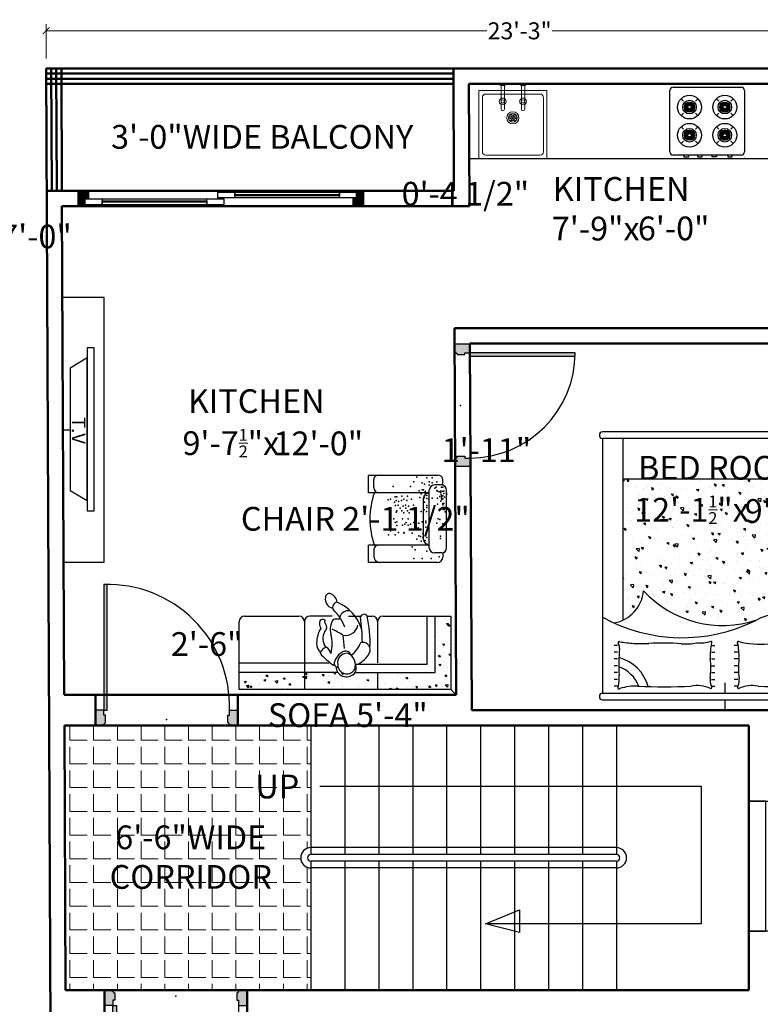
# Model space of a CAD drawing. Units: inches. Extents: x 4508 to 5907, y 877 to 1592.
# Tile 19 of 20: x 5566 to 5784, y 1298 to 1588. Entities that reach past the tile are written whole.
import ezdxf

# ---------------------------------------------------------------- set-up
doc = ezdxf.new("R2010")
doc.units = ezdxf.units.IN
doc.layers.get('DEFPOINTS').update_dxf_attribs({"color": 8})
for name, color, linetype, lineweight in [('A-ANNO-DIMS', 2, 'Continuous', 18), ('A-ANNO-TEXT', 7, 'Continuous', 25), ('A-DOOR', 4, 'Continuous', 25), ('A-EQPM', 6, 'Continuous', 25), ('A-FLOR-CASE', 30, 'Continuous', 25), ('A-FLOR-FIXT', 8, 'Continuous', 18), ('A-FLOR-PATT', 252, 'Continuous', 13), ('A-FLOR-STRS', 5, 'Continuous', 25), ('A-FURN', 24, 'Continuous', 18), ('A-WALL', 7, 'Continuous', 50)]:
    doc.layers.add(name, color=color, linetype=linetype, lineweight=lineweight)
doc.layers.add('doors & windows', color=30, linetype='Continuous')
doc.layers.add('furniture', color=24, linetype='Continuous')
doc.styles.get("Standard").update_dxf_attribs({"font": 'arial.ttf'})
doc.dimstyles.new('details', dxfattribs={"dimtxt": 5, "dimasz": 2, "dimexe": 2, "dimexo": 3, "dimgap": 1, "dimtad": 0, "dimdec": 1, "dimzin": 0, "dimdsep": 46, "dimlunit": 4, "dimtxsty": 'Standard', "dimblk": 'ARCHTICK', "dimcen": 3, "dimclrd": 256, "dimclre": 256, "dimclrt": 256, "dimadec": 0, "dimazin": 0, "dimtfac": 0.5, "dimtdec": 1, "dimtofl": 0, "dimtmove": 0, "dimatfit": 3, "dimldrblk": 'CLOSEDBLANK', "dimfxl": 2, "dimtolj": 1, "dimtzin": 0, "dimlwd": -1, "dimlwe": -1, "dimarcsym": 0})
doc.dimstyles.new('text', dxfattribs={"dimtxt": 7, "dimasz": 0, "dimexe": 3, "dimexo": 3, "dimgap": 0, "dimtad": 1, "dimtih": 1, "dimtoh": 1, "dimzin": 3, "dimdsep": 46, "dimlunit": 4, "dimtxsty": 'Standard', "dimblk": 'CLOSEDBLANK', "dimcen": 3, "dimse1": 1, "dimse2": 1, "dimsd1": 1, "dimsd2": 1, "dimclrd": 256, "dimclre": 256, "dimclrt": 256, "dimadec": 0, "dimazin": 0, "dimtfac": 0.5, "dimtofl": 0, "dimtmove": 0, "dimatfit": 3, "dimfxl": 3, "dimtolj": 1, "dimtzin": 0, "dimlwd": -1, "dimlwe": -1, "dimarcsym": 0})

# ---------------------------------------------------------------- blocks, each defined once
blk = doc.blocks.new('*D114')
at = {"layer": 'DEFPOINTS', "color": 0, "transparency": 16777216}
for p in [(5615.84, 1381.24), (5615.84, 1303.24), (5616.61, 1303.24)]:
    blk.add_point(p, dxfattribs=at)
at = {"layer": 'A-ANNO-DIMS', "color": 0, "transparency": 16777216, "insert": (5616.61, 1341.61), "char_height": 7, "attachment_point": 5}
blk.add_mtext('\\A1;6\'-6"WIDE \\PCORRIDOR', dxfattribs=at)
blk = doc.blocks.new('_ClosedBlank')
at = {"color": 0, "lineweight": -2}
for p, q in [((-1, 0.17), (0, 0)), ((-1, 0.17), (-1, -0.17)), ((0, 0), (-1, -0.17))]:
    blk.add_line(p, q, dxfattribs=at)
blk = doc.blocks.new('FD')
h = blk.add_hatch()
h.set_pattern_fill('ANSI31', color=256, style=0)
h.set_pattern_definition([(315, (2e-11, -5), (-0.0883883, -0.0883883), [])])
h.paths.add_polyline_path([(0, -4.5), (0, 0), (3, 0), (3, -2.5), (2, -2.5), (2, -4), (2, -4.5)])
h = blk.add_hatch()
h.set_pattern_fill('ANSI31', color=256, style=0)
h.set_pattern_definition([(135, (84, 0.5), (0.0883883, 0.0883883), [])])
h.paths.add_polyline_path([(84, 0), (84, -4.5), (81, -4.5), (81, -2), (82, -2), (82, -0.5), (82, 0)])
for p, q in [((0, -4.5), (0, 0)), ((0, 0), (84, 0)), ((84, 0), (84, -4.5)), ((0, -4.5), (84, -4.5))]:
    blk.add_line(p, q)
at = {"layer": 'doors & windows'}
for p, q in [((0, 0), (3, 0)), ((82, 0), (84, 0)), ((82, -2), (82, 0)), ((2, -2.5), (2, -4)), ((2, -2.5), (2, -4.5)), ((76.94, -1.25), (46.1, -1.25)), ((82, -2), (82, -0.5)), ((2, -4.5), (0, -4.5)), ((7.06, -3.25), (37.9, -3.25)), ((84, -4.5), (81, -4.5))]:
    blk.add_line(p, q, dxfattribs=at)
for points in [[(3, 0), (3, -2.5), (2, -2.5)], [(2, -4), (43, -4), (43, -2.5), (2, -2.5), (2, -4)], [(7.06, -2.5), (7.06, -4), (7.06, -3), (37.9, -3), (37.9, -4), (37.9, -2.5)], [(82, -0.5), (41, -0.5), (41, -2), (82, -2), (82, -0.5)], [(76.94, -2), (76.94, -0.5), (76.94, -1.5), (46.1, -1.5), (46.1, -0.5), (46.1, -2)], [(81, -4.5), (81, -2), (82, -2)]]:
    blk.add_lwpolyline(points, dxfattribs=at)
blk = doc.blocks.new('*D117')
at = {"layer": 'DEFPOINTS', "color": 0, "transparency": 16777216}
for p in [(5791.67, 1535.67), (5698.68, 1533.69), (5791.67, 1523.15)]:
    blk.add_point(p, dxfattribs=at)
at = {"layer": 'A-ANNO-DIMS', "color": 0, "transparency": 16777216, "insert": (5735.91, 1532.61), "char_height": 7, "attachment_point": 5}
blk.add_mtext('\\A1;       KITCHEN\\P7\'-9"x', dxfattribs=at)
blk = doc.blocks.new('*D118')
at = {"layer": 'DEFPOINTS', "color": 0, "transparency": 16777216}
for p in [(5748.26, 1569.42), (5758.87, 1569.42), (5754.78, 1497.42)]:
    blk.add_point(p, dxfattribs=at)
at = {"layer": 'A-ANNO-DIMS', "color": 0, "transparency": 16777216, "insert": (5758.87, 1526.82), "char_height": 7, "attachment_point": 5}
blk.add_mtext('\\A1;6\'-0"', dxfattribs=at)
blk = doc.blocks.new('stove')
at = {"layer": 'furniture'}
h = blk.add_hatch(dxfattribs=at)
h.set_pattern_fill('HEX', color=256, angle=180, style=0)
h.set_pattern_definition([(360, (22, 21.5), (1e-16, 0.2165064), [0.125, -0.25]), (120, (22, 21.5), (-0.1875, -0.1082532), [0.125, -0.25]), (60, (22.125, 21.5), (-0.1875, 0.1082532), [0.125, -0.25])])
h.paths.add_polyline_path([(5.36, 16.21, 1), (8.36, 16.21, 1)])
h.paths.add_polyline_path([(7.36, 16.21, -1), (6.36, 16.21, -1)], flags=16)
h = blk.add_hatch(dxfattribs=at)
h.set_pattern_fill('HEX', color=256, angle=180, style=0)
h.set_pattern_definition([(180, (2e-13, 21.5), (-1e-16, 0.2165064), [0.125, -0.25]), (60, (2e-13, 21.5), (0.1875, -0.1082532), [0.125, -0.25]), (120, (-0.125, 21.5), (0.1875, 0.1082532), [0.125, -0.25])])
h.paths.add_polyline_path([(13.64, 16.21, 1), (16.64, 16.21, 1)])
h.paths.add_polyline_path([(15.64, 16.21, -1), (14.64, 16.21, -1)], flags=16)
h = blk.add_hatch(dxfattribs=at)
h.set_pattern_fill('HEX', color=256, angle=180, style=0)
h.set_pattern_definition([(360, (22, 0.5), (-1e-16, -0.2165064), [0.125, -0.25]), (240, (22, 0.5), (-0.1875, 0.1082532), [0.125, -0.25]), (300, (22.125, 0.5), (-0.1875, -0.1082532), [0.125, -0.25])])
h.paths.add_polyline_path([(8.36, 5.79, 1), (5.36, 5.79, 1)])
h.paths.add_polyline_path([(6.36, 5.79, -1), (7.36, 5.79, -1)], flags=16)
h = blk.add_hatch(dxfattribs=at)
h.set_pattern_fill('HEX', color=256, angle=180, style=0)
h.set_pattern_definition([(180, (2e-13, 0.5), (1e-16, -0.2165064), [0.125, -0.25]), (300, (2e-13, 0.5), (0.1875, 0.1082532), [0.125, -0.25]), (240, (-0.125, 0.5), (0.1875, -0.1082532), [0.125, -0.25])])
h.paths.add_polyline_path([(16.64, 5.79, 1), (13.64, 5.79, 1)])
h.paths.add_polyline_path([(14.64, 5.79, -1), (15.64, 5.79, -1)], flags=16)
for p, q in [((1, 1), (1, 21)), ((2, 22), (20, 22)), ((21, 21), (21, 1)), ((1, 17.86), (0.5, 17.86)), ((0.5, 17.86), (0.5, 16.36)), ((4.39, 18.69), (5.1, 17.98)), ((8.63, 17.98), (9.34, 18.69)), ((13.37, 17.98), (12.66, 18.69)), ((17.61, 18.69), (16.9, 17.98)), ((0.5, 16.36), (1, 16.36)), ((0.5, 13.8), (0.5, 12.5)), ((1, 13.8), (0.5, 13.8)), ((0.5, 12.5), (1, 12.5)), ((4.39, 13.74), (5.1, 14.45)), ((8.63, 14.45), (9.34, 13.74)), ((13.37, 14.45), (12.66, 13.74)), ((17.61, 13.74), (16.9, 14.45)), ((0.5, 9.5), (1, 9.5)), ((0.5, 8.2), (0.5, 9.5)), ((1, 8.2), (0.5, 8.2)), ((4.39, 8.26), (5.1, 7.55)), ((8.63, 7.55), (9.34, 8.26)), ((13.37, 7.55), (12.66, 8.26)), ((17.61, 8.26), (16.9, 7.55)), ((0.5, 4.94), (0.5, 3.64)), ((1, 4.94), (0.5, 4.94)), ((0.5, 3.64), (1, 3.64)), ((4.39, 3.31), (5.1, 4.02)), ((8.63, 4.02), (9.34, 3.31)), ((13.37, 4.02), (12.66, 3.31)), ((17.61, 3.31), (16.9, 4.02)), ((20, 0), (2, 0))]:
    blk.add_line(p, q, dxfattribs=at)
for centre, radius in [((6.86, 16.21), 3.5), ((6.86, 16.21), 2), ((6.86, 16.21), 1.5), ((15.14, 16.21), 3.5), ((15.14, 16.21), 2), ((15.14, 16.21), 1.5), ((6.86, 16.21), 0.5), ((15.14, 16.21), 0.5), ((6.86, 5.79), 3.5), ((15.14, 5.79), 3.5), ((6.86, 5.79), 2), ((6.86, 5.79), 1.5), ((6.86, 5.79), 0.5), ((15.14, 5.79), 2), ((15.14, 5.79), 1.5), ((15.14, 5.79), 0.5)]:
    blk.add_circle(centre, radius, dxfattribs=at)
for centre, start, end in [((2, 21), 90, 180), ((20, 21), 0, 90), ((2, 1), 180, 270), ((20, 1), 270, 0)]:
    blk.add_arc(centre, 1, start, end, dxfattribs=at)
at = {"layer": 'furniture', "ltscale": 9}
blk.add_point((0, 0), dxfattribs=at)
blk = doc.blocks.new('sink')
for p, q in [((0, 0), (-24, 0)), ((0, 0), (0, 0)), ((-22, -3), (-2, -3)), ((-22, -23), (-22, -3)), ((-21, -21), (-21, -5)), ((-20, -4), (-4, -4)), ((-3, -5), (-3, -21)), ((-2, -3), (-2, -23)), ((-0.5, -9.5), (-7.5, -9.5)), ((-0.5, -10.5), (-7.5, -10.5)), ((-0.5, -9.5), (-0.5, -10.5)), ((0, -9), (0, -11)), ((-0.5, -15.5), (-7.5, -15.5)), ((-0.5, -16.5), (-7.5, -16.5)), ((-0.5, -15.5), (-0.5, -16.5)), ((0, -15), (0, -17)), ((-22, -23), (-2, -23)), ((-20, -22), (-4, -22))]:
    blk.add_line(p, q)
for centre, radius in [((-10, -13), 1.79), ((-5.18, -10), 1), ((-5.18, -10), 0.5), ((-10, -13), 1.29), ((-10.66, -12.62), 0.25), ((-10.66, -13.38), 0.25), ((-10, -12.24), 0.25), ((-10, -13), 0.25), ((-10, -13.76), 0.25), ((-9.34, -12.62), 0.25), ((-9.34, -13.38), 0.25), ((-5.18, -16), 1), ((-5.18, -16), 0.5)]:
    blk.add_circle(centre, radius)
for centre, radius, start, end in [((-20, -5), 1, 90, 180), ((-4, -5), 1, 0, 90), ((-7.5, -10), 0.5, 90, 270), ((0.01, -9.51), 0.511, 91.1728, 178.8272), ((0.01, -10.49), 0.511, 181.1728, 268.8272), ((-7.5, -16), 0.5, 90, 270), ((0.01, -15.51), 0.511, 91.1728, 178.8272), ((0.01, -16.49), 0.511, 181.1728, 268.8272), ((-20, -21), 1, 180, 270), ((-4, -21), 1, 270, 0)]:
    blk.add_arc(centre, radius, start, end)
blk = doc.blocks.new('_ArchTick')
at = {"color": 0, "linetype": 'ByBlock', "const_width": 0.15}
blk.add_lwpolyline([(-0.5, -0.5), (0.5, 0.5)], dxfattribs=at)
blk = doc.blocks.new('*D121')
at = {"layer": 'A-ANNO-DIMS', "color": 0, "transparency": 16777216}
for p, q in [((5573.99, 1576.92), (5573.99, 1587.03)), ((5852.99, 1576.92), (5852.99, 1587.03)), ((5573.99, 1585.03), (5703.86, 1585.03)), ((5852.99, 1585.03), (5723.12, 1585.03))]:
    blk.add_line(p, q, dxfattribs=at)
at = {"layer": 'DEFPOINTS', "color": 0, "transparency": 16777216}
for p in [(5852.99, 1585.03), (5573.99, 1573.92), (5852.99, 1573.92)]:
    blk.add_point(p, dxfattribs=at)
at = {"layer": 'A-ANNO-DIMS', "color": 0, "transparency": 16777216, "xscale": 2, "yscale": 2, "zscale": 2, "rotation": 180}
blk.add_blockref('_ArchTick', (5573.99, 1585.03), dxfattribs=at)
at = {"layer": 'A-ANNO-DIMS', "color": 0, "transparency": 16777216, "xscale": 2, "yscale": 2, "zscale": 2}
blk.add_blockref('_ArchTick', (5852.99, 1585.03), dxfattribs=at)
at = {"layer": 'A-ANNO-DIMS', "color": 0, "transparency": 16777216, "insert": (5713.49, 1585.03), "char_height": 5, "attachment_point": 5}
blk.add_mtext('\\A1;23\'-3"', dxfattribs=at)
blk = doc.blocks.new('*D122')
at = {"layer": 'DEFPOINTS', "color": 0, "transparency": 16777216}
for p in [(5620.3, 1573.92), (5622.07, 1537.92), (5637.65, 1537.92)]:
    blk.add_point(p, dxfattribs=at)
at = {"layer": 'A-ANNO-DIMS', "color": 0, "transparency": 16777216, "insert": (5637.65, 1553.8), "char_height": 7, "attachment_point": 5}
blk.add_mtext('\\A1;3\'-0"WIDE BALCONY', dxfattribs=at)
blk = doc.blocks.new('*D123')
at = {"layer": 'DEFPOINTS', "color": 0, "transparency": 16777216}
for p in [(5792.26, 1492.92), (5759.25, 1384.92), (5790.34, 1384.92)]:
    blk.add_point(p, dxfattribs=at)
at = {"layer": 'A-ANNO-DIMS', "color": 0, "transparency": 16777216, "insert": (5790.34, 1443.57), "char_height": 7, "attachment_point": 5}
blk.add_mtext('\\A1;9\'-0"', dxfattribs=at)
blk = doc.blocks.new('*D124')
at = {"layer": 'DEFPOINTS', "color": 0, "transparency": 16777216}
for p in [(5715.67, 1442.67), (5861.17, 1442.67), (5861.17, 1439.77)]:
    blk.add_point(p, dxfattribs=at)
at = {"layer": 'A-ANNO-DIMS', "color": 0, "transparency": 16777216, "insert": (5764.12, 1449.77), "char_height": 7, "attachment_point": 5}
blk.add_mtext('\\A1;        BED ROOM\\P12\'-1{\\H0.5x;\\S1/2;}"x', dxfattribs=at)
blk = doc.blocks.new('bed')
at = {"layer": 'furniture'}
h = blk.add_hatch(dxfattribs=at)
h.set_pattern_fill('AR-CONC', color=256, angle=-90, style=0)
h.set_pattern_definition([(320, (0, 2.38), (-0.6275, -7.1726), [0.75, -8.25]), (265, (0, 2.38), (7.5219, 1.3875), [0.6, -6.6]), (10.451, (-0.052, 1.782), (6.8944, -5.7851), [0.6374, -7.0114]), (316.184, (2, 2.38), (-1.6552, -10.6724), [1.125, -12.375]), (6.636, (1.862, 1.491), (9.7412, -9.3466), [0.9561, -10.5171]), (261.184, (2, 2.38), (9.7412, -9.3466), [0.9, -9.9]), (291, (1.5, 1.38), (-4.0262, -5.96907), [0.75, -8.25]), (236, (1.5, 1.38), (7.2515, -2.43315), [0.6, -6.6]), (341.451, (1.1645, 0.8826), (3.2253, -8.4022), [0.6374, -7.0114]), (307.5, (0, 2.38), (3.32894, -0.1216), [0, -6.52, 0, -6.7, 0, -6.625]), (277.5, (0, 2.38), (3.94412, -2.6307), [0, -3.82, 0, -6.37, 0, -2.525]), (237.5, (0, 4.61), (-0.22555, -5.33822), [0, -2.5, 0, -7.8, 0, -10.35]), (227.5, (0, 5.61), (1.00105, -5.83186), [0, -3.25, 0, -5.18, 0, -7.35])])
h.paths.add_polyline_path([(30.01, -68), (30.01, -26.5, 0.263043), (23.9, -35.15, 0.293424), (-9.18, -26.47, -0.156683), (-23.39, -28.72), (-23.39, -68)])
for p, q in [((0, -3), (0, 0)), ((36.01, -3), (-36.01, -3)), ((-36.01, -5), (-36.01, -80)), ((36.01, -5), (-36.01, -5)), ((0, -8), (0, -5)), ((36.01, -80), (36.01, -5)), ((-31.24, -7.07), (-32.24, -7.07)), ((-3.81, -7.07), (-2.81, -7.07)), ((3.89, -7.07), (2.89, -7.07)), ((31.63, -7.07), (32.63, -7.07)), ((-31.24, -9.07), (-32.24, -9.07)), ((-31.24, -11.07), (-32.24, -11.07)), ((-3.81, -9.07), (-2.81, -9.07)), ((-3.81, -11.07), (-2.81, -11.07)), ((3.89, -9.07), (2.89, -9.07)), ((3.89, -11.07), (2.89, -11.07)), ((31.63, -9.07), (32.63, -9.07)), ((31.63, -11.07), (32.63, -11.07)), ((-31.24, -13.07), (-32.24, -13.07)), ((-3.81, -13.07), (-2.81, -13.07)), ((3.89, -13.07), (2.89, -13.07)), ((31.63, -13.07), (32.63, -13.07)), ((-31.24, -15.07), (-32.24, -15.07)), ((-31.24, -17.07), (-32.24, -17.07)), ((-3.81, -15.07), (-2.81, -15.07)), ((-3.81, -17.07), (-2.81, -17.07)), ((3.89, -15.07), (2.89, -15.07)), ((3.89, -17.07), (2.89, -17.07)), ((31.63, -15.07), (32.63, -15.07)), ((31.63, -17.07), (32.63, -17.07)), ((-31.24, -19.07), (-32.24, -19.07)), ((-3.81, -19.07), (-2.81, -19.07)), ((3.89, -19.07), (2.89, -19.07)), ((31.63, -19.07), (32.63, -19.07)), ((-36.01, -80), (36.01, -80)), ((-36.01, -82), (36.01, -82))]:
    blk.add_line(p, q, dxfattribs=at)
at = {"layer": 'furniture', "ltscale": 5}
blk.add_line((-30.01, -26.66), (-30.01, -80), dxfattribs=at)
at = {"layer": 'furniture', "ltscale": 0.3}
for p, q in [((-23.39, -80), (-23.39, -28.72)), ((-30.01, -68), (30.01, -68))]:
    blk.add_line(p, q, dxfattribs=at)
at = {"layer": 'furniture', "ltscale": 7}
blk.add_line((30.01, -80), (30.01, -26.5), dxfattribs=at)
at = {"layer": 'furniture'}
for centre, radius, start, end in [((-35.95, -4), 1, 93.3831, 266.6169), ((35.95, -4), 1, 273.3831, 86.6169), ((-31.1, -6.57), 0.382, 35.8976, 208.6272), ((-44.44, -13.85), 14.82, 27.1629, 28.6272), ((-46.76, -9.65), 15.72, 357.4804, 9.3956), ((-34.45, -3.51), 9.85, 289.8695, 338.9843), ((-34.45, -3.51), 12.47, 286.0319, 344.1205), ((-26.35, 6.68), 13.76, 251.1782, 273.3982), ((-18.02, -163.6), 156.72, 87.0032, 92.7497), ((-8.03, 2.03), 9.29, 258.896, 294.7184), ((0.25, -8.8), 4.49, 159.0146, 186.273), ((-4.03, -6.67), 0.282, 335.7259, 114.303), ((3.22, -9.94), 7.68, 155.7259, 159.0146), ((4.11, -6.67), 0.282, 65.697, 204.2741), ((-3.14, -9.94), 7.68, 20.9854, 24.2741), ((-0.17, -8.8), 4.49, 353.727, 20.9854), ((8.12, 2.03), 9.29, 245.2816, 281.104), ((18.1, -163.6), 156.72, 87.2503, 92.9968), ((34.54, -3.51), 12.47, 195.8795, 253.9681), ((34.54, -3.51), 9.85, 201.0157, 250.1305), ((26.43, 6.68), 13.76, 266.6018, 288.8218), ((31.18, -6.57), 0.382, 331.3728, 144.1024), ((46.84, -9.65), 15.72, 170.6044, 182.5196), ((44.53, -13.85), 14.82, 151.3728, 152.8371), ((-28.62, 31.03), 42.31, 266.4836, 266.6487), ((54.88, -13.16), 85.99, 178.1209, 183.3613), ((-32.82, -12.44), 28.78, 354.3784, 6.273), ((32.9, -12.44), 28.78, 173.727, 185.6216), ((-54.8, -13.16), 85.99, 356.6387, 1.8791), ((28.7, 31.03), 42.31, 273.3513, 273.5164), ((12.28, -16.11), 16.48, 177.0317, 192.8678), ((-12.19, -16.11), 16.48, 347.1322, 2.9683), ((-31.05, -19.91), 0.291, 147.6219, 311.9343), ((-33.2, -18.55), 2.25, 327.6219, 339.2246), ((-34.13, -18.41), 3.18, 342.7809, 3.755), ((-24.4, -58.01), 38.42, 93.5164, 99.6766), ((-24.52, -56.06), 36.48, 86.4836, 93.5164), ((-18.49, 70.49), 90.23, 267.5921, 273.6329), ((-10.31, -44.95), 25.52, 75.952, 95.5452), ((-3.95, -19.99), 0.265, 231.9005, 52.8902), ((4.03, -19.99), 0.265, 127.1098, 308.0995), ((7.57, -34.68), 14.87, 87.3976, 103.1191), ((11.44, -34.81), 15.32, 84.694, 102.0355), ((18.57, 70.49), 90.23, 266.3671, 272.4079), ((24.6, -56.06), 36.48, 86.4836, 93.5164), ((24.48, -58.01), 38.42, 80.3234, 86.4836), ((31.13, -19.91), 0.291, 228.0657, 32.3781), ((34.21, -18.41), 3.18, 176.245, 197.2191), ((33.28, -18.55), 2.25, 200.7754, 212.3781), ((-19.79, -5.47), 23.53, 226.4061, 297.4441), ((12.51, -69.71), 48.38, 60.9345, 116.3227), ((0.6, -56.57), 31.65, 42.5874, 108.5034), ((34.61, -36.23), 10.76, 101.1719, 174.259), ((-35.95, -81), 1, 93.3831, 266.6169), ((35.95, -81), 1, 273.3831, 86.6169)]:
    blk.add_arc(centre, radius, start, end, dxfattribs=at)
blk = doc.blocks.new('tv')
at = {"layer": 'furniture'}
blk.add_line((0, 0), (2, 0), dxfattribs=at)
for points in [[(0, -39), (12, -39), (12, 39), (0, 39)], [(7, 24.19), (7, -23.81), (9, -23.81), (9, 24.19), (7, 24.19)]]:
    blk.add_lwpolyline(points, dxfattribs=at)
blk.add_lwpolyline([(7, -20.81), (7, 21.19), (2, 18.19), (2, -17.81)], close=True, dxfattribs=at)
blk.add_text('T.V', height=4, rotation=270, dxfattribs=at).set_placement((2.46, 3.81))
blk = doc.blocks.new('MD')
at = {"layer": 'doors & windows'}
h = blk.add_hatch(dxfattribs=at)
h.set_pattern_fill('DOTS', color=256, scale=2, style=0)
h.set_pattern_definition([(180, (0, -4), (-0.0625, 0.125), [0, -0.125])])
h.paths.add_polyline_path([(2.5, 37), (3.5, 37), (3.5, 0), (2.5, 0)])
h = blk.add_hatch(dxfattribs=at)
h.set_pattern_fill('DOTS', color=256, scale=2, style=0)
h.set_pattern_definition([(0, (0, -0.5), (0.0625, 0.125), [0, -0.125])])
h.paths.add_polyline_path([(42, -4.5), (42, 0), (39.5, 0), (39.5, -1.5), (39, -1.5), (39, -3.75), (39.25, -3.75, 0.403966), (39.75, -4.25), (39.75, -4.5)])
h.paths.add_polyline_path([(0, -4.5), (2.25, -4.5), (2.25, -4.25, 0.403966), (2.75, -3.75), (3, -3.75), (3, -1.5), (2.5, -1.5), (2.5, 0), (0, 0)])
for p, q in [((0, 0), (0, -4.5)), ((42, 0), (42, -4.5))]:
    blk.add_line(p, q)
blk.add_line((0, -4.5), (2.25, -4.5), dxfattribs=at)
blk.add_lwpolyline([(3.5, 0), (3.5, 37), (2.5, 37), (2.5, 0)], close=True, dxfattribs=at)
for points in [[(3, -3.75), (3, -1.5), (2.5, -1.5), (2.5, 0), (0, 0)], [(39, -3.75), (39, -1.5), (39.5, -1.5), (39.5, 0), (42, 0)], [(42, -4.5), (39.75, -4.5)]]:
    blk.add_lwpolyline(points, dxfattribs=at)
for points in [[(2.25, -4.5), (2.25, -4.25, 0.403966), (2.75, -3.75), (3, -3.75)], [(39.75, -4.5), (39.75, -4.25, -0.403966), (39.25, -3.75), (39, -3.75)]]:
    blk.add_lwpolyline(points, format="xyb", dxfattribs=at)
at = {"layer": 'doors & windows', "ltscale": 6}
blk.add_arc((3.73, 1.23), 35.79, 358.0281, 91.9719, dxfattribs=at)
at = {"layer": 'doors & windows'}
blk.add_point((21, -2.75), dxfattribs=at)
blk = doc.blocks.new('MAN')
at = {"layer": 'doors & windows'}
blk.add_line((1.3, -9.85), (0.89, -5.45), dxfattribs=at)
for centre, radius, start, end in [((0.1, 0.48), 3.6, 2.8928, 134.5528), ((-0.36, -7.56), 8.07, 108.0153, 157.5724), ((-0.81, 1.3), 2.37, 132.7993, 210.1219), ((1.3, 0.05), 4.16, 155.2349, 248.5051), ((0, 0), 3.06, 359.7942, 144.0351), ((-0.98, 0.55), 5.34, 289.2819, 356.6237), ((2.86, -0.44), 1.38, 352.7443, 87.7525), ((-8.99, -19.77), 24.04, 41.647, 56.3067), ((4.14, -10.82), 9.46, 125.6851, 158.6987), ((0.38, -2.75), 1.79, 192.3382, 283.0231), ((-0.1, -0.61), 3.22, 267.7788, 10.6507), ((-5.32, -4.92), 2.54, 170.002, 284.7527), ((34.75, -7.19), 42.53, 177.9613, 192.4551), ((15.87, -7.04), 10.97, 162.7002, 196.7262), ((8.59, -3.01), 3.29, 193.5598, 239.9446), ((5.83, -2.73), 3.32, 289.6374, 341.2911), ((3.84, -8.67), 4.24, 325.4363, 41.8446), ((6.12, -7.03), 4.01, 358.2671, 46.939), ((54.76, -7.35), 59.95, 180.1044, 188.2297), ((0.5, -14.05), 4.27, 79.2575, 168.509), ((16.49, 13.41), 27.78, 236.8487, 245.427), ((-0.78, -6.94), 10.91, 330.7562, 358.8997), ((9.03, -7.36), 14.72, 197.1765, 246.7641), ((12.84, -8.62), 12.77, 197.9012, 229.3504), ((-0.19, -11.81), 5.78, 325.2412, 16.1794), ((8.85, -12.54), 2.12, 136.0875, 215.1077), ((7.06, -13.61), 2.15, 328.4119, 38.6474), ((-5.78, -15.61), 1.25, 217.214, 345.0614), ((-0.4, -15.27), 2.81, 261.6005, 345.5998), ((3.21, -8.72), 6.53, 262.8142, 281.931), ((6.8, -14.37), 0.689, 315.9836, 61.7947), ((8.05, -14.12), 1.05, 224.0636, 323.687), ((3.09, -19.2), 1.68, 274.444, 31.8659), ((4.09, -22.01), 3.16, 349.15, 77.9716), ((6.99, -20.36), 3.8, 187.9766, 248.0432), ((5.75, -22.44), 1.45, 262.6631, 353.5986)]:
    blk.add_arc(centre, radius, start, end, dxfattribs=at)
blk = doc.blocks.new('sofa 2')
at = {"layer": 'furniture', "ltscale": 0.5}
h = blk.add_hatch(dxfattribs=at)
h.set_pattern_fill('AR-CONC', color=256, angle=450, style=0)
h.set_pattern_definition([(40, (-1099.1507, 871.655), (-0.627521, 7.172602), [0.75, -8.25]), (95, (-1099.151, 871.655), (7.52192, -1.387513), [0.6, -6.6]), (349.5486, (-1099.203, 872.253), (6.894395, 5.785094), [0.637402, -7.01142]), (43.8158, (-1097.151, 871.655), (-1.65519, 10.67241), [1.125, -12.375]), (353.3644, (-1097.289, 872.544), (9.74118, 9.34663), [0.9561, -10.51713]), (98.8158, (-1097.151, 871.655), (9.74119, 9.34662), [0.9, -9.9]), (69, (-1097.6507, 872.655), (-4.02619, 5.96907), [0.75, -8.25]), (124, (-1097.651, 872.655), (7.2515, 2.433153), [0.6, -6.6]), (18.5486, (-1097.986, 873.1524), (3.225305, 8.402226), [0.637402, -7.01142]), (52.5, (-1099.1507, 871.655), (3.3289385, 0.1215986), [0, -6.52, 0, -6.7, 0, -6.625]), (82.5, (-1099.1507, 871.655), (3.944117, 2.630695), [0, -3.82, 0, -6.37, 0, -2.525]), (122.5, (-1099.1507, 869.425), (-0.2255487, 5.3382244), [0, -2.5, 0, -7.8, 0, -10.35]), (132.5, (-1099.1507, 868.425), (1.00105, 5.831862), [0, -3.25, 0, -5.18, 0, -7.35])])
h.paths.add_polyline_path([(-8.27, -37.7, 0.168872), (-7.9, -36.76, 0.613808), (-6.95, -30.77, 0.074869), (-8.27, -30.38), (-8.27, -29), (-2, -29), (-2, -56), (-8.27, -56)])
h.paths.add_polyline_path([(-8.27, -7.77), (-29, -7.77), (-29, -2), (-2, -2), (-2, -29), (-8.27, -29)])
h.paths.add_polyline_path([(-8.27, -80), (-2, -80), (-2, -56), (-8.27, -56)])
at = {"layer": 'furniture'}
for p, q in [((-2, -2), (0, 0)), ((-29, -2), (-2, -2)), ((-29, -27), (-29, -2)), ((-2, -2), (-2, -80)), ((-8.27, -7.77), (-29, -7.77)), ((-11.27, -10.77), (-29, -10.77)), ((-11.27, -37.27), (-11.27, -10.77)), ((-8.27, -37.27), (-8.27, -7.77)), ((-27, -29), (-11.8, -29)), ((-8.27, -29), (-2, -29)), ((-29, -32.87), (-29, -31)), ((-29, -39.74), (-29, -35.16)), ((-8.27, -37.7), (-8.27, -37.7)), ((-29, -45.8), (-29, -54)), ((-11.8, -80), (-11.8, -46.89)), ((-8.27, -43.66), (-8.27, -80)), ((-29, -78), (-29, -58)), ((-27, -56), (-2, -56)), ((-2, -80), (-27, -80))]:
    blk.add_line(p, q, dxfattribs=at)
for centre, start, end in [((-27, -27), 180, 270), ((-27, -31), 90, 180), ((-27, -54), 180, 270), ((-27, -58), 90, 180), ((-27, -78), 180, 270)]:
    blk.add_arc(centre, 2, start, end, dxfattribs=at)
at = {"xscale": 1.099999999999999, "yscale": 1.099999999999999, "zscale": 1.099999999999999, "rotation": 270}
blk.add_blockref('MAN', (-11.13, -40.34), dxfattribs=at)
blk = doc.blocks.new('sofa')
at = {"layer": 'furniture'}
for p, q in [((3.13, 15.05), (27, 15.05)), ((27, 15.05), (27, 9.05)), ((1.33, 11.75), (1.33, 13.25)), ((1.8, 11.75), (4.13, 11.75)), ((25.2, 10.85), (25.2, 12.75)), ((0, 9.95), (0, -9.95)), ((6, 9.95), (6, -9.95)), ((6, 9.05), (27, 9.05)), ((8, 7.25), (8, -7.25)), ((8, 4.04), (8, 3.89)), ((6.03, -9.05), (27, -9.05)), ((27, -9.05), (27, -15.05)), ((1.33, -11.75), (1.33, -13.65)), ((1.8, -11.75), (4.13, -11.75)), ((25.2, -10.85), (25.2, -13.65)), ((3.13, -15.05), (27, -15.05))]:
    blk.add_line(p, q, dxfattribs=at)
for centre, radius, start, end in [((3.13, 13.25), 1.8, 90, 180), ((22.91, 12.82), 2.29, 358.3453, 77.7487), ((1.8, 9.95), 1.8, 90, 180), ((1.8, 9.95), 1.8, 90, 180), ((4.14, 9.89), 1.86, 1.747, 90.2901), ((4.14, 9.89), 1.86, 1.747, 90.2901), ((23.4, 10.85), 1.8, 270, 0), ((5.91, 6.93), 2.12, 8.589, 87.4366), ((-0.79, 0), 27.33, 340.6621, 19.3379), ((1.8, -9.95), 1.8, 180, 270), ((4.14, -9.89), 1.86, 269.7099, 358.253), ((5.96, -6.99), 2.06, 272.0036, 352.7589), ((23.4, -10.85), 1.8, 0, 90), ((2.83, -13.59), 1.5, 182.4941, 281.7559), ((23.7, -13.59), 1.5, 258.2441, 357.5059)]:
    blk.add_arc(centre, radius, start, end, dxfattribs=at)
for p in [(5.3, 13.66), (8.48, 13.66), (11.4, 13.66), (0.72, 11.51), (2.64, 13.13), (6.89, 11.2), (10.87, 10.67), (6.8, 8.68), (7.42, 7.45), (8.85, 7.66), (10.28, 7.04), (11.93, 9.61), (2.09, 5.95), (2.11, 6.75), (6.8, 6.43), (7.42, 5.82), (8.24, 6.43), (8.24, 5), (9.05, 6.02), (9.67, 5.82), (11.92, 4.9), (14.64, 4.9), (14.78, 4.7), (16.69, 4.7), (17.83, 5.52), (19.47, 4.09), (20.08, 5.52), (0.72, 1.97), (1.3, 1.71), (1.32, 3.3), (2.38, 0.24), (3.44, 1.44), (7.21, 2.86), (7.21, 1.39), (7.21, 0.82), (8.03, 2.04), (8.44, 0.98), (9.67, 1.43), (9.87, 3.06), (10.49, 0.98), (11.31, 1.19), (12.53, 1.84), (13.35, 2.21), (13.35, 0.01), (14.03, 1.19), (14.44, 1.84), (15.26, 2.21), (15.26, 0.01), (17.21, 2.25), (17.24, 1.02), (17.85, 1.19), (19.26, 1.19), (0.5, -2.45), (0.72, -3.25), (1.26, -3.25), (2.11, -3.25), (2.64, -2.98), (2.91, -0.01), (7.01, -2.55), (7.83, -3.16), (8.85, -2.55), (12.94, -2.14), (13.56, -2.75), (14.85, -2.14), (15.46, -2.75), (17.21, -2.75), (17.44, -2.34), (18.24, -0.03), (1.03, -5.36), (1.32, -5.36), (1.36, -4.83), (1.62, -6.69), (2.05, -6.16), (3.17, -5.1), (6.8, -3.98), (6.8, -4.59), (7.62, -5.82), (10.49, -3.77), (11.51, -4.79), (13.15, -4.38), (13.76, -6.43), (14.17, -3.77), (14.23, -4.79), (15.05, -4.38), (15.66, -6.43), (16.07, -3.77), (16.6, -6.02), (16.8, -4.79), (17.44, -6.43), (17.65, -4.59), (18.06, -5.82), (20.28, -6.63), (-0.03, -8.54), (0.77, -7.48), (0.99, -9.6), (1.03, -8.81), (1.36, -6.95), (1.36, -8.01), (1.56, -8.01), (1.58, -9.6), (1.79, -6.95), (1.79, -7.48), (1.85, -8.28), (2.05, -9.07), (2.09, -9.6), (2.38, -7.75), (2.64, -9.34), (3.17, -7.22), (3.17, -9.6), (3.44, -9.87), (5.03, -7.22), (6.19, -6.84), (6.39, -8.88), (6.8, -7.04), (6.8, -8.06), (7.42, -8.88), (7.42, -9.49), (7.83, -7.25), (7.83, -7.86), (8.03, -10.11), (8.44, -10.11), (8.85, -8.68), (9.26, -7.45), (9.46, -9.7), (12.12, -6.84), (13.56, -7.86), (14.85, -6.84), (15.46, -7.86), (17.24, -7.65), (17.83, -7.65), (19.47, -6.84), (1.3, -10.93), (1.79, -10.93), (3.38, -12.78), (3.64, -10.93), (4.09, -10.66), (5.03, -12.52), (6.09, -11.72), (6.09, -12.78), (7.69, -11.99), (8.48, -12.52), (11.4, -12.78), (12.46, -11.19), (18.51, -11.19), (5.03, -14.17), (6.89, -14.17), (10.34, -14.44)]:
    blk.add_point(p, dxfattribs=at)
blk = doc.blocks.new('D1')
at = {"layer": 'doors & windows'}
h = blk.add_hatch(dxfattribs=at)
h.set_pattern_fill('DOTS', color=256, scale=2, angle=180, style=0)
h.set_pattern_definition([(180, (-2e-12, -4), (-0.0625, -0.125), [0, -0.125])])
h.paths.add_polyline_path([(2.5, 0), (3.5, 0), (3.5, 30.98, 0.008066), (2.5, 31)])
h = blk.add_hatch(dxfattribs=at)
h.set_pattern_fill('DOTS', color=256, scale=2, angle=180, style=0)
h.set_pattern_definition([(180, (0, -0.5), (-0.0625, -0.125), [0, -0.125])])
h.paths.add_polyline_path([(0, -4.5), (2.25, -4.5), (2.25, -4.25, 0.403966), (2.75, -3.75), (3, -3.75), (3, -1.5), (2.5, -1.5), (2.5, 0), (0, 0)])
h.paths.add_polyline_path([(36, -4.5), (36, 0), (33.5, 0), (33.5, -1.5), (33, -1.5), (33, -3.75), (33.25, -3.75, 0.403966), (33.75, -4.25), (33.75, -4.5)])
for p, q in [((0, 0), (0, -4.5)), ((36, 0), (36, -4.5))]:
    blk.add_line(p, q)
blk.add_lwpolyline([(3.5, 0), (3.5, 31), (2.5, 31), (2.5, 0)], close=True, dxfattribs=at)
for points in [[(3, -3.75), (3, -1.5), (2.5, -1.5), (2.5, 0), (0, 0)], [(33, -3.75), (33, -1.5), (33.5, -1.5), (33.5, 0), (36, 0)], [(0, -4.5), (2.25, -4.5)], [(36, -4.5), (33.75, -4.5)]]:
    blk.add_lwpolyline(points, dxfattribs=at)
for points in [[(2.25, -4.5), (2.25, -4.25, 0.403966), (2.75, -3.75), (3, -3.75)], [(33.75, -4.5), (33.75, -4.25, -0.403966), (33.25, -3.75), (33, -3.75)]]:
    blk.add_lwpolyline(points, format="xyb", dxfattribs=at)
at = {"layer": 'doors & windows', "ltscale": 6}
blk.add_arc((2.5, 0), 31, 0, 90, dxfattribs=at)
at = {"layer": 'doors & windows'}
blk.add_point((18, -2.75), dxfattribs=at)
blk = doc.blocks.new('*D125')
at = {"layer": 'DEFPOINTS', "color": 0, "transparency": 16777216}
for p in [(5579, 1463.46), (5694.55, 1459.35), (5694.55, 1453.58)]:
    blk.add_point(p, dxfattribs=at)
at = {"layer": 'A-ANNO-DIMS', "color": 0, "transparency": 16777216, "insert": (5628.42, 1469.4), "char_height": 7, "attachment_point": 5}
blk.add_mtext('\\A1;       KITCHEN\\P9\'-7{\\H0.5x;\\S1/2;}"x', dxfattribs=at)
blk = doc.blocks.new('*D126')
at = {"layer": 'DEFPOINTS', "color": 0, "transparency": 16777216}
for p in [(5644.95, 1533.42), (5654.2, 1533.42), (5647.3, 1389.42)]:
    blk.add_point(p, dxfattribs=at)
at = {"layer": 'A-ANNO-DIMS', "color": 0, "transparency": 16777216, "insert": (5654.2, 1463.5), "char_height": 7, "attachment_point": 5}
blk.add_mtext('\\A1;12\'-0"', dxfattribs=at)
blk = doc.blocks.new('*D150')
at = {"layer": 'DEFPOINTS', "color": 0, "transparency": 16777216}
for p in [(5583.45, 1533.42), (5667.45, 1533.42), (5667.45, 1520.82)]:
    blk.add_point(p, dxfattribs=at)
at = {"layer": 'A-ANNO-DIMS', "transparency": 16777216, "insert": (5537.21, 1524.44), "char_height": 7, "attachment_point": 5}
blk.add_mtext('\\A1;SLIDING DOOR 7\'-0"', dxfattribs=at)
blk = doc.blocks.new('*D151')
at = {"layer": 'DEFPOINTS', "color": 0, "transparency": 16777216}
for p in [(5667.45, 1537.92), (5680.05, 1537.92), (5667.45, 1533.42)]:
    blk.add_point(p, dxfattribs=at)
at = {"layer": 'A-ANNO-DIMS', "transparency": 16777216, "insert": (5697.51, 1537.04), "char_height": 7, "attachment_point": 5}
blk.add_mtext('\\A1;0\'-4 1/2"', dxfattribs=at)
blk = doc.blocks.new('*D176')
at = {"layer": 'DEFPOINTS', "color": 0, "transparency": 16777216}
for p in [(5668.95, 1454.14), (5665.09, 1428.42), (5668.95, 1428.42)]:
    blk.add_point(p, dxfattribs=at)
at = {"layer": 'A-ANNO-DIMS', "transparency": 16777216, "insert": (5665.09, 1441.28), "char_height": 7, "attachment_point": 5}
blk.add_mtext('\\A1;CHAIR 2\'-1 1/2"', dxfattribs=at)
blk = doc.blocks.new('*D177')
at = {"layer": 'DEFPOINTS', "color": 0, "transparency": 16777216}
for p in [(5668.95, 1458), (5668.95, 1454.14), (5692.02, 1454.14)]:
    blk.add_point(p, dxfattribs=at)
at = {"layer": 'A-ANNO-DIMS', "transparency": 16777216, "insert": (5703.71, 1461.51), "char_height": 7, "attachment_point": 5}
blk.add_mtext('\\A1;1\'-11"', dxfattribs=at)
blk = doc.blocks.new('*D180')
at = {"layer": 'DEFPOINTS', "color": 0, "transparency": 16777216}
for p in [(5630.89, 1389.42), (5694.84, 1389.42), (5694.84, 1379.82)]:
    blk.add_point(p, dxfattribs=at)
at = {"layer": 'A-ANNO-DIMS', "transparency": 16777216, "insert": (5662.87, 1383.44), "char_height": 7, "attachment_point": 5}
blk.add_mtext('\\A1;SOFA 5\'-4"', dxfattribs=at)
blk = doc.blocks.new('*D181')
at = {"layer": 'DEFPOINTS', "color": 0, "transparency": 16777216}
for p in [(5630.89, 1419.36), (5621.29, 1389.42), (5630.89, 1389.42)]:
    blk.add_point(p, dxfattribs=at)
at = {"layer": 'A-ANNO-DIMS', "transparency": 16777216, "insert": (5621.29, 1404.39), "char_height": 7, "attachment_point": 5}
blk.add_mtext('\\A1;2\'-6"', dxfattribs=at)
blk = doc.blocks.new('*D191')
at = {"layer": 'DEFPOINTS', "color": 0, "transparency": 16777216}
for p in [(5539.438529, 1302.416611), (5579.745522, 1302.416611), (5579.787188, 1293.416611)]:
    blk.add_point(p, dxfattribs=at)
at = {"layer": 'A-ANNO-DIMS', "transparency": 16777216, "insert": (5539.438529, 1297.916611), "char_height": 7, "attachment_point": 5}
blk.add_mtext('\\A1;0\'-9"', dxfattribs=at)

msp = doc.modelspace()

# ---------------------------------------------------------------- hatches: boundary and pattern name
at = {"layer": 'A-FLOR-PATT'}
h = msp.add_hatch(dxfattribs=at)
h.set_pattern_fill('ANGLE', color=256)
h.set_pattern_definition([(0, (0, 0), (0, 6.985), [5.08, -1.905]), (90, (0, 0), (-6.985, 4e-16), [5.08, -1.905])])
h.paths.add_polyline_path([(5651.989, 1338.417, -1), (5651.989, 1344.417), (5651.989, 1380.417), (5579.384, 1380.417), (5579.746, 1302.417), (5651.989, 1302.417)])
h.paths.add_polyline_path([(5588.063, 1328.497), (5644.803, 1328.497), (5644.803, 1354.665), (5588.063, 1354.665)], flags=24)
h.paths.add_polyline_path([(5633.846, 1357.01), (5650.991, 1357.01), (5650.991, 1367.689), (5633.846, 1367.689)], flags=24)

# ---------------------------------------------------------------- linework, layer by layer
at = {"layer": 'A-EQPM'}
msp.add_lwpolyline([(5789.989, 1319.79), (5780.989, 1319.79), (5785.989, 1319.79), (5785.989, 1358.075), (5780.989, 1358.075), (5789.989, 1358.075), (5787.989, 1358.075), (5787.989, 1319.79)], dxfattribs=at)
at = {"layer": 'A-FLOR-CASE'}
msp.add_line((5698.511, 1547.417), (5795.989, 1547.417), dxfattribs=at)
at = {"layer": 'A-FLOR-STRS'}
for p, q in [((5651.989, 1380.417), (5651.989, 1342.417)), ((5661.989, 1380.417), (5661.989, 1342.417)), ((5671.989, 1380.417), (5671.989, 1342.417)), ((5681.989, 1380.417), (5681.989, 1342.417)), ((5691.989, 1380.417), (5691.989, 1342.417)), ((5701.989, 1380.417), (5701.989, 1342.417)), ((5711.989, 1380.417), (5711.989, 1342.417)), ((5721.989, 1380.417), (5721.989, 1342.417)), ((5731.989, 1380.417), (5731.989, 1342.417)), ((5741.989, 1380.417), (5741.989, 1342.417)), ((5741.989, 1344.417), (5651.989, 1344.417)), ((5741.989, 1342.417), (5651.989, 1342.417)), ((5741.989, 1340.417), (5651.989, 1340.417)), ((5651.989, 1340.417), (5651.989, 1302.417)), ((5661.989, 1340.417), (5661.989, 1302.417)), ((5671.989, 1340.417), (5671.989, 1302.417)), ((5681.989, 1340.417), (5681.989, 1302.417)), ((5691.989, 1340.417), (5691.989, 1302.417)), ((5701.989, 1340.417), (5701.989, 1302.417)), ((5711.989, 1340.417), (5711.989, 1302.417)), ((5721.989, 1340.417), (5721.989, 1302.417)), ((5731.989, 1340.417), (5731.989, 1302.417)), ((5741.989, 1340.417), (5741.989, 1302.417)), ((5741.989, 1338.417), (5651.989, 1338.417))]:
    msp.add_line(p, q, dxfattribs=at)
msp.add_lwpolyline([(5654.641, 1362.49), (5766.971, 1362.49), (5766.971, 1321.99), (5703.475, 1321.99), (5713.475, 1326.119), (5713.475, 1319.442), (5703.475, 1321.99)], dxfattribs=at)
for centre, radius, start, end in [((5651.989, 1341.417), 3, 90, 270), ((5741.989, 1341.417), 3, 270, 90), ((5651.989, 1341.417), 1, 90, 270), ((5741.989, 1341.417), 1, 270, 90)]:
    msp.add_arc(centre, radius, start, end, dxfattribs=at)
at = {"layer": 'A-WALL'}
for p, q in [((5573.989, 1573.917), (5854.266, 1573.917)), ((5576.989, 925.917), (5573.989, 1573.917)), ((5574.009, 1572.417), (5694.011, 1572.417)), ((5575.655, 1537.903), (5575.489, 1573.917)), ((5577.155, 1537.91), (5576.989, 1573.917)), ((5578.655, 1537.917), (5578.489, 1573.917)), ((5694.156, 1537.917), (5693.99, 1573.917)), ((5574.009, 1570.917), (5694.011, 1570.917)), ((5574.009, 1569.417), (5694.011, 1569.417)), ((5698.511, 1569.417), (5795.989, 1569.417)), ((5698.677, 1533.417), (5698.511, 1569.417)), ((5574.155, 1537.917), (5694.156, 1537.917)), ((5578.676, 1533.417), (5698.677, 1533.417)), ((5579.343, 1389.417), (5578.676, 1533.417)), ((5694.344, 1497.417), (5795.989, 1497.417)), ((5694.844, 1389.417), (5694.344, 1497.417)), ((5698.865, 1492.917), (5848.489, 1492.917)), ((5699.365, 1384.917), (5698.865, 1492.917)), ((5579.343, 1389.417), (5694.844, 1389.417)), ((5588.501, 1380.417), (5588.501, 1389.417)), ((5630.501, 1380.417), (5630.501, 1389.417)), ((5699.365, 1384.917), (5848.489, 1384.917)), ((5579.384, 1380.417), (5780.989, 1380.417)), ((5579.746, 1302.417), (5579.384, 1380.417)), ((5780.989, 1380.417), (5780.989, 1302.417)), ((5579.746, 1302.417), (5780.989, 1302.417)), ((5591.171, 1293.417), (5591.171, 1302.417)), ((5633.198, 1302.417), (5633.198, 1293.417))]:
    msp.add_line(p, q, dxfattribs=at)

# ---------------------------------------------------------------- block references
at = {"layer": 'A-DOOR'}
for name, p in [('FD', (5583.45, 1537.917)), ('MD', (5588.501, 1384.917))]:
    msp.add_blockref(name, p, dxfattribs=at)
at = {"layer": 'A-DOOR', "rotation": 270}
msp.add_blockref('D1', (5698.866, 1492.686), dxfattribs=at)
at = {"layer": 'A-DOOR', "xscale": -1, "rotation": 180}
msp.add_blockref('MD', (5591.198, 1297.931), dxfattribs=at)
at = {"layer": 'A-FLOR-FIXT', "rotation": 90}
for name, p in [('sink', (5698.511, 1569.417)), ('stove', (5779.738, 1547.417))]:
    msp.add_blockref(name, p, dxfattribs=at)
at = {"layer": 'A-FURN'}
msp.add_blockref('tv', (5579.119, 1467.46), dxfattribs=at)
at = {"layer": 'A-FURN', "rotation": 180}
msp.add_blockref('bed', (5773.927, 1384.917), dxfattribs=at)
at = {"layer": 'A-FURN'}
for name, p, xscale, yscale, zscale, rotation in [('sofa', (5691.996, 1441.242), 0.8518887825114443, 0.8518887825114443, 0.8518887825114443, 180), ('sofa 2', (5694.844, 1389.417), 0.7994643722202431, 0.7994643722202431, 0.7994643722202431, 270)]:
    msp.add_blockref(name, p, dxfattribs=dict(at, xscale=xscale, yscale=yscale, zscale=zscale, rotation=rotation))

# ---------------------------------------------------------------- texts
at = {"layer": 'A-ANNO-TEXT'}
msp.add_text('UP', height=7, dxfattribs=at).set_placement((5635.626, 1358.909))

# ---------------------------------------------------------------- dimensions: what is measured, and where the dimension line sits
at = {"layer": 'A-ANNO-DIMS'}
dim = msp.add_linear_dim(base=(5852.989, 1585.029), p1=(5573.989, 1573.917), p2=(5852.989, 1573.917), dimstyle='details', override={"dimclrd": 0, "dimclre": 0, "dimclrt": 0}, dxfattribs=at)
dim.commit()
dim.dimension.update_dxf_attribs({"geometry": '*D121', "text_midpoint": (5713.489, 1585.029)})
for base, p1, p2, text, override, picture, middle in [((5637.649, 1537.917), (5620.299, 1573.917), (5622.07, 1537.917), '<>WIDE BALCONY', {"dimtad": 0, "dimclrd": 0, "dimclre": 0, "dimclrt": 0}, '*D122', (5637.649, 1553.798)), ((5616.614, 1303.24), (5615.841, 1381.24), (5615.841, 1303.24), '<>WIDE \\PCORRIDOR', {"dimclrd": 0, "dimclre": 0, "dimclrt": 0}, '*D114', (5616.614, 1341.607))]:
    dim = msp.add_linear_dim(base=base, p1=p1, p2=p2, angle=90, text=text, dimstyle='text', override=override, dxfattribs=at)
    dim.commit()
    dim.dimension.update_dxf_attribs({"geometry": picture, "text_midpoint": middle, "dimtype": 160})
for base, p1, p2, picture, middle in [((5758.872, 1569.417), (5754.785, 1497.417), (5748.259, 1569.417), '*D118', (5758.872, 1526.817)), ((5654.202, 1533.417), (5647.297, 1389.417), (5644.95, 1533.417), '*D126', (5654.202, 1463.497)), ((5790.337, 1384.917), (5792.265, 1492.917), (5759.245, 1384.917), '*D123', (5790.337, 1443.573))]:
    dim = msp.add_linear_dim(base=base, p1=p1, p2=p2, angle=90, dimstyle='text', override={"dimclrd": 0, "dimclre": 0, "dimclrt": 0}, dxfattribs=at)
    dim.commit()
    dim.dimension.update_dxf_attribs({"geometry": picture, "text_midpoint": middle, "dimtype": 160})
for base, p1, p2, text, picture, middle in [((5791.668, 1523.146), (5698.676, 1533.691), (5791.668, 1535.667), '       KITCHEN\\P<>x', '*D117', (5735.911, 1523.146)), ((5694.547, 1459.346), (5579, 1463.455), (5694.547, 1453.582), '       KITCHEN\\P<>x', '*D125', (5628.423, 1459.346)), ((5861.167, 1439.773), (5715.667, 1442.667), (5861.167, 1442.667), '        BED ROOM\\P<>x', '*D124', (5764.115, 1439.773))]:
    dim = msp.add_linear_dim(base=base, p1=p1, p2=p2, text=text, dimstyle='text', override={"dimclrd": 0, "dimclre": 0, "dimclrt": 0}, dxfattribs=at)
    dim.commit()
    dim.dimension.update_dxf_attribs({"geometry": picture, "text_midpoint": middle, "dimtype": 160})
for base, p1, p2, angle, override, picture, middle in [((5680.05, 1537.917), (5667.45, 1533.417), (5667.45, 1537.917), 90, {"dimdec": 1, "dimrnd": 0, "dimzin": 1, "dimlunit": 4, "dimfrac": 2}, '*D151', (5697.509, 1537.036)), ((5668.947, 1457.997), (5692.019, 1454.139), (5668.947, 1454.139), 180, {"dimdec": 1, "dimrnd": 0, "dimzin": 1, "dimlunit": 4, "dimfrac": 2}, '*D177', (5703.713, 1461.511)), ((5621.293, 1389.417), (5630.887, 1419.358), (5630.887, 1389.417), 270, {"dimdec": 1, "dimrnd": 0, "dimzin": 1, "dimlunit": 4, "dimfrac": 2}, '*D181', (5621.293, 1404.387)), ((5539.439, 1302.417), (5579.787, 1293.417), (5579.746, 1302.417), 90, {"dimdec": 1, "dimlfac": 1, "dimrnd": 0, "dimzin": 1, "dimdsep": 46, "dimlunit": 4, "dimfrac": 2}, '*D191', (5539.439, 1297.917))]:
    dim = msp.add_linear_dim(base=base, p1=p1, p2=p2, angle=angle, dimstyle='text', override=override, dxfattribs=at)
    dim.commit()
    dim.dimension.update_dxf_attribs({"geometry": picture, "text_midpoint": middle})
for base, p1, p2, text, picture, middle in [((5667.45, 1520.817), (5583.45, 1533.417), (5667.45, 1533.417), 'SLIDING DOOR <>', '*D150', (5537.214, 1524.438)), ((5694.844, 1379.823), (5630.887, 1389.417), (5694.844, 1389.417), 'SOFA <>', '*D180', (5662.865, 1383.445))]:
    dim = msp.add_linear_dim(base=base, p1=p1, p2=p2, text=text, dimstyle='text', override={"dimdec": 1, "dimrnd": 0, "dimzin": 1, "dimlunit": 4, "dimfrac": 2}, dxfattribs=at)
    dim.commit()
    dim.dimension.update_dxf_attribs({"geometry": picture, "text_midpoint": middle})
dim = msp.add_linear_dim(base=(5665.089, 1428.42), p1=(5668.947, 1454.139), p2=(5668.947, 1428.42), angle=270, text='CHAIR <>', dimstyle='text', override={"dimdec": 1, "dimrnd": 0, "dimzin": 1, "dimlunit": 4, "dimfrac": 2}, dxfattribs=at)
dim.commit()
dim.dimension.update_dxf_attribs({"geometry": '*D176', "text_midpoint": (5665.089, 1441.28)})

doc.saveas('drawing.dxf')
